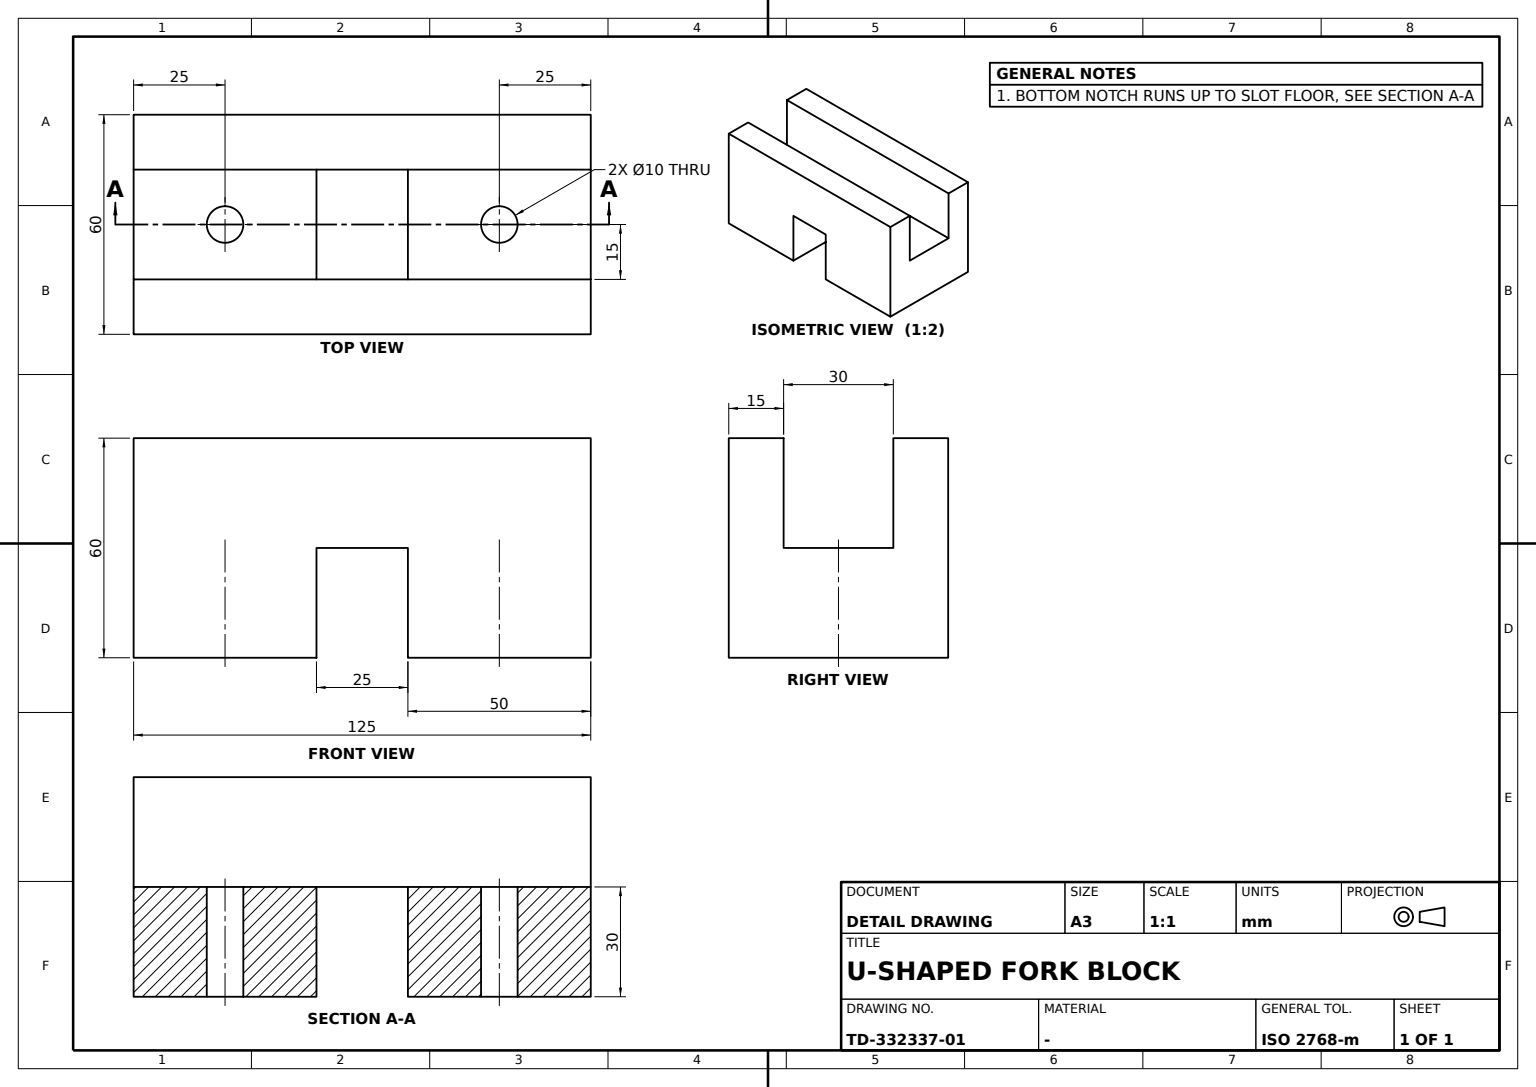
CATIA V5 part; units mm, degrees
sketch "Sketch1" plane through (0, 0, 0) normal (1, 0, 0) x (0, 1, 0)
  line L0 (-62.5, 0) -> (-12.5, 0)
  point P0 (-62.5, 0)
  point P1 (62.5, 0)
  line L1 (-62.5, 0) -> (-62.5, 60)
  line L2 (-62.5, 60) -> (62.5, 60)
  line L3 (62.5, 60) -> (62.5, 0)
  line L4 (-12.5, 0) -> (-12.5, 30)
  line L5 (-12.5, 30) -> (12.5, 30)
  line L6 (12.5, 30) -> (12.5, 0)
  point P2 (12.5, 0)
  line L7 (12.5, 0) -> (62.5, 0)
  dimension "length L1" = 60
  dimension "distance L3 L6" = 50
  dimension "distance L6 L4" = 25
  dimension "distance L5 L0" = 30
  dimension "distance P0 P1" = 125
  constraint horizontal L0 x-axis
  constraint horizontal L2 x-axis
  constraint horizontal L5 x-axis
  constraint horizontal L7 x-axis
  constraint vertical L1 y-axis
  constraint vertical L3 y-axis
  constraint vertical L4 y-axis
  constraint vertical L6 y-axis
  constraint coincidence P2 L0
  constraint coincidence L0 origin
  constraint coincidence L0 L7
  constraint equidistance P0 P1 origin
extrude "Pad1" add sketch "Sketch1" along normal mid plane 60
sketch "Sketch2" plane through (0, 62.5, 0) normal (0, 1, 0) x (-1, 0, 0)
  line L0 (-15, 72.2289) -> (15, 72.2289)
  line L1 (15, 72.2289) -> (15, 30)
  line L2 (15, 30) -> (-15, 30)
  line L3 (-15, 30) -> (-15, 72.2289)
  line L4 (30, 0) -> (30, 60) construction
  line L5 (-30, 0) -> (-30, 60) construction
  line L6 (30, 0) -> (-30, 0) construction
  dimension "distance L4 L1" = 15
  dimension "distance L3 L5" = 15
  dimension "distance L6 L2" = 30
  constraint horizontal L0 x-axis
  constraint horizontal L2 x-axis
  constraint vertical L1 y-axis
  constraint vertical L3 y-axis
extrude "Pocket1" cut sketch "Sketch2" against normal through all
sketch "Sketch3" plane through (0, 0, 30) normal (0, 0, 1) x (1, 0, 0)
  circle A0 centre (0, -37.5) radius 5
  point P0 (0, -37.5)
  point P1 (0, -42.5)
  point P2 (0, 37.5)
  circle A1 centre (0, 37.5) radius 5
  dimension "radius A0" = 5
  dimension "distance P0 P2" = 75
  constraint coincidence P0 y-axis
  constraint coincidence A0 P1
  constraint coincidence P1 y-axis
  constraint symmetry A0 A1 x-axis
extrude "Pocket2" cut sketch "Sketch3" against normal through all
properties part number "U-Shaped Fork Bracket with Double Mounting Holes"
